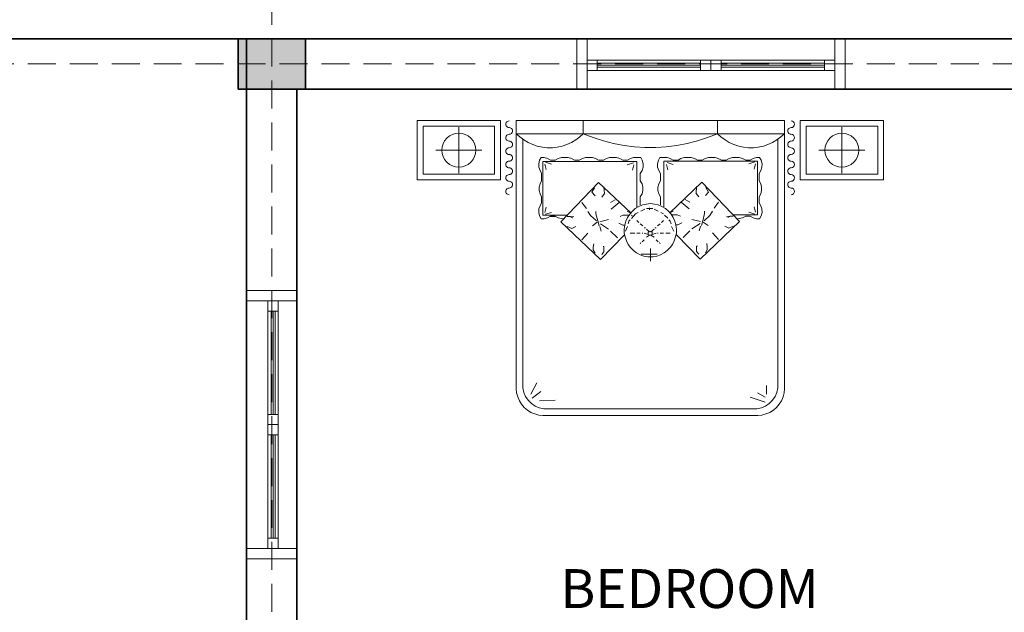
# Model space of a CAD drawing. Units: inches. Extents: x 782 to 2660, y -1008 to 166.
# Tile 8 of 12: x 1058 to 1234, y -58 to 48. Entities that reach past the tile are written whole.
import ezdxf

# ---------------------------------------------------------------- set-up
doc = ezdxf.new("R2010")
doc.units = ezdxf.units.IN
doc.header["$MEASUREMENT"] = 0
doc.linetypes.add('DASHED', pattern=[0.75, 0.5, -0.25])
for name, color, linetype, lineweight in [('A-ANNO-DIMS', 4, 'Continuous', 18), ('A-AREA-IDEN', 4, 'Continuous', 18), ('A-COLS', 7, 'Continuous', 35), ('A-FURN', 8, 'Continuous', 13), ('A-Glaz', 4, 'Continuous', 18), ('A-GRID', 8, 'DASHED', 13), ('A-WALL', 7, 'Continuous', 35)]:
    doc.layers.add(name, color=color, linetype=linetype, lineweight=lineweight)
doc.styles.get("Standard").update_dxf_attribs({"font": 'arial.ttf'})
doc.dimstyles.get("Standard").update_dxf_attribs({"dimtxt": 5, "dimasz": 2, "dimexe": 0.18, "dimexo": 0.0625, "dimgap": 0.09, "dimtad": 0, "dimtih": 1, "dimtoh": 1, "dimdec": 0, "dimzin": 0, "dimdsep": 46, "dimlunit": 3, "dimtxsty": 'Standard', "dimblk": 'ARCHTICK', "dimcen": 0.09, "dimadec": 0, "dimazin": 0, "dimtfac": 1, "dimtdec": 0, "dimtofl": 0, "dimtmove": 0, "dimatfit": 3, "dimfxl": 1, "dimtolj": 1, "dimtzin": 0, "dimarcsym": 0})

# ---------------------------------------------------------------- blocks, each defined once
blk = doc.blocks.new('d-bed-4')
at = {"color": 0, "linetype": 'ByBlock'}
for p, q in [((0.56, 0), (0, 0)), ((0, 0), (0, -0.4)), ((0.56, -0.4), (0.56, 0)), ((0.6639, -1.8), (0.6639, 0)), ((0.6639, 0), (2.4639, 0)), ((0.6639, 0), (2.4639, 0)), ((0.6639, -1.8), (0.6639, 0)), ((1.1139, 0), (1.1139, -0.09)), ((2.0139, 0), (2.0139, -0.09)), ((2.4639, 0), (2.4639, -1.8)), ((2.4639, 0), (2.4639, -1.8)), ((2.5679, -0.4), (2.5679, 0)), ((2.5679, 0), (3.1279, 0)), ((3.1279, 0), (3.1279, -0.4)), ((0.52, -0.04), (0.04, -0.04)), ((0.04, -0.04), (0.04, -0.36)), ((0.28, -0.0461), (0.28, -0.3539)), ((0.52, -0.36), (0.52, -0.04)), ((2.6079, -0.36), (2.6079, -0.04)), ((2.6079, -0.04), (3.0879, -0.04)), ((2.8479, -0.0461), (2.8479, -0.3539)), ((3.0879, -0.04), (3.0879, -0.36)), ((2.4639, -0.09), (0.6639, -0.09)), ((0.6639, -0.09), (0.6891, -0.1116)), ((0.6891, -0.1116), (0.7161, -0.1314)), ((0.7089, -1.7946), (0.7089, -0.1278)), ((0.7161, -0.1314), (0.7449, -0.1476)), ((1.0347, -0.1476), (1.0635, -0.1314)), ((1.0635, -0.1314), (1.0905, -0.1116)), ((1.0905, -0.1116), (1.1139, -0.09)), ((1.1139, -0.09), (1.1805, -0.1152)), ((1.1805, -0.1152), (1.2489, -0.1368)), ((1.8789, -0.1368), (1.9473, -0.1152)), ((1.9473, -0.1152), (2.0139, -0.09)), ((2.0139, -0.09), (2.0373, -0.1116)), ((2.0373, -0.1116), (2.0643, -0.1314)), ((2.0643, -0.1314), (2.0931, -0.1476)), ((2.3829, -0.1476), (2.4117, -0.1314)), ((2.4117, -0.1314), (2.4387, -0.1116)), ((2.4189, -0.1278), (2.4189, -1.7946)), ((2.4387, -0.1116), (2.4639, -0.09)), ((0.7449, -0.1476), (0.7755, -0.162)), ((0.7755, -0.162), (0.8061, -0.1728)), ((0.8061, -0.1728), (0.8403, -0.18)), ((0.8403, -0.18), (0.8727, -0.1836)), ((0.8727, -0.1836), (0.9069, -0.1836)), ((0.9069, -0.1836), (0.9393, -0.18)), ((0.9393, -0.18), (0.9717, -0.1728)), ((0.9717, -0.1728), (1.0041, -0.162)), ((1.0041, -0.162), (1.0347, -0.1476)), ((1.2489, -0.1368), (1.3173, -0.1548)), ((1.3173, -0.1548), (1.3875, -0.1692)), ((1.3875, -0.1692), (1.4577, -0.1782)), ((1.4577, -0.1782), (1.5279, -0.1818)), ((1.5279, -0.1818), (1.5999, -0.1818)), ((1.5999, -0.1818), (1.6701, -0.1782)), ((1.6701, -0.1782), (1.7403, -0.1692)), ((1.7403, -0.1692), (1.8105, -0.1548)), ((1.8105, -0.1548), (1.8789, -0.1368)), ((2.0931, -0.1476), (2.1237, -0.162)), ((2.1237, -0.162), (2.1561, -0.1728)), ((2.1561, -0.1728), (2.1885, -0.18)), ((2.1885, -0.18), (2.2209, -0.1836)), ((2.2209, -0.1836), (2.2551, -0.1836)), ((2.2551, -0.1836), (2.2875, -0.18)), ((2.2875, -0.18), (2.3217, -0.1728)), ((2.3217, -0.1728), (2.3523, -0.162)), ((2.3523, -0.162), (2.3829, -0.1476)), ((0.1261, -0.2), (0.4339, -0.2)), ((0.8205, -0.2682), (0.8313, -0.2484)), ((0.8313, -0.2484), (0.8529, -0.2484)), ((0.8529, -0.2484), (0.8745, -0.2556)), ((0.8745, -0.2556), (0.8943, -0.2664)), ((0.9249, -0.2664), (0.9465, -0.2556)), ((0.9465, -0.2556), (0.9681, -0.2502)), ((0.9681, -0.2502), (0.9897, -0.2484)), ((0.9897, -0.2484), (1.0131, -0.2502)), ((1.0131, -0.2502), (1.0347, -0.2556)), ((1.0347, -0.2556), (1.0563, -0.2664)), ((1.0869, -0.2664), (1.1085, -0.2556)), ((1.1085, -0.2556), (1.1301, -0.2502)), ((1.1301, -0.2502), (1.1517, -0.2484)), ((1.1517, -0.2484), (1.1751, -0.2502)), ((1.1751, -0.2502), (1.1967, -0.2556)), ((1.1967, -0.2556), (1.2165, -0.2664)), ((1.2489, -0.2664), (1.2687, -0.2556)), ((1.2687, -0.2556), (1.2903, -0.2502)), ((1.2903, -0.2502), (1.3137, -0.2484)), ((1.3137, -0.2484), (1.3371, -0.2502)), ((1.3371, -0.2502), (1.3587, -0.2556)), ((1.3587, -0.2556), (1.3785, -0.2664)), ((1.4109, -0.2664), (1.4307, -0.2556)), ((1.4307, -0.2556), (1.4505, -0.2484)), ((1.4505, -0.2484), (1.4739, -0.2484)), ((1.4739, -0.2484), (1.5009, -0.2484)), ((1.5009, -0.2484), (1.5099, -0.2682)), ((1.6269, -0.2484), (1.6179, -0.2682)), ((1.6539, -0.2484), (1.6269, -0.2484)), ((1.6773, -0.2484), (1.6539, -0.2484)), ((1.6971, -0.2556), (1.6773, -0.2484)), ((1.7169, -0.2664), (1.6971, -0.2556)), ((1.7691, -0.2556), (1.7493, -0.2664)), ((1.7907, -0.2502), (1.7691, -0.2556)), ((1.8141, -0.2484), (1.7907, -0.2502)), ((1.8375, -0.2502), (1.8141, -0.2484)), ((1.8591, -0.2556), (1.8375, -0.2502)), ((1.8789, -0.2664), (1.8591, -0.2556)), ((1.9311, -0.2556), (1.9113, -0.2664)), ((1.9527, -0.2502), (1.9311, -0.2556)), ((1.9761, -0.2484), (1.9527, -0.2502)), ((1.9977, -0.2502), (1.9761, -0.2484)), ((2.0193, -0.2556), (1.9977, -0.2502)), ((2.0409, -0.2664), (2.0193, -0.2556)), ((2.0931, -0.2556), (2.0715, -0.2664)), ((2.1147, -0.2502), (2.0931, -0.2556)), ((2.1381, -0.2484), (2.1147, -0.2502)), ((2.1597, -0.2502), (2.1381, -0.2484)), ((2.1813, -0.2556), (2.1597, -0.2502)), ((2.2029, -0.2664), (2.1813, -0.2556)), ((2.2533, -0.2556), (2.2335, -0.2664)), ((2.2749, -0.2484), (2.2533, -0.2556)), ((2.2965, -0.2484), (2.2749, -0.2484)), ((2.3073, -0.2682), (2.2965, -0.2484)), ((3.0018, -0.2), (2.6939, -0.2)), ((0.8151, -0.2916), (0.8205, -0.2682)), ((0.8169, -0.315), (0.8151, -0.2916)), ((0.8241, -0.3366), (0.8169, -0.315)), ((0.8439, -0.6354), (0.8439, -0.2754)), ((0.8439, -0.2754), (1.4721, -0.2754)), ((0.8565, -0.2934), (0.8655, -0.3294)), ((0.8619, -0.2808), (0.9015, -0.2934)), ((0.8943, -0.2664), (0.9249, -0.2664)), ((1.0563, -0.2664), (1.0869, -0.2664)), ((1.2165, -0.2664), (1.2489, -0.2664)), ((1.3785, -0.2664), (1.4109, -0.2664)), ((1.4505, -0.2844), (1.4091, -0.2988)), ((1.4541, -0.2988), (1.4451, -0.3348)), ((1.4721, -0.2754), (1.4721, -0.5814)), ((1.5153, -0.315), (1.5081, -0.3366)), ((1.5099, -0.2682), (1.5153, -0.2916)), ((1.5153, -0.2916), (1.5153, -0.315)), ((1.6179, -0.2682), (1.6125, -0.2916)), ((1.6125, -0.2916), (1.6125, -0.315)), ((1.6125, -0.315), (1.6197, -0.3366)), ((2.2821, -0.2736), (1.6539, -0.2736)), ((1.6539, -0.2736), (1.6539, -0.5796)), ((1.6719, -0.297), (1.6809, -0.333)), ((1.6755, -0.2826), (1.7169, -0.297)), ((1.7493, -0.2664), (1.7169, -0.2664)), ((1.9113, -0.2664), (1.8789, -0.2664)), ((2.0715, -0.2664), (2.0409, -0.2664)), ((2.2335, -0.2664), (2.2029, -0.2664)), ((2.2641, -0.279), (2.2245, -0.2916)), ((2.2695, -0.2916), (2.2605, -0.3276)), ((2.2821, -0.6336), (2.2821, -0.2736)), ((2.3037, -0.3366), (2.3109, -0.315)), ((2.3127, -0.2916), (2.3073, -0.2682)), ((2.3109, -0.315), (2.3127, -0.2916)), ((0.04, -0.36), (0.52, -0.36)), ((0.8349, -0.3564), (0.8241, -0.3366)), ((0.8349, -0.405), (0.8349, -0.3564)), ((1.5081, -0.3366), (1.4955, -0.3564)), ((1.4955, -0.3564), (1.4955, -0.405)), ((1.6197, -0.3366), (1.6323, -0.3564)), ((1.6323, -0.3564), (1.6323, -0.405)), ((2.2929, -0.3564), (2.3037, -0.3366)), ((2.2929, -0.405), (2.2929, -0.3564)), ((3.0879, -0.36), (2.6079, -0.36)), ((0, -0.4), (0.56, -0.4)), ((0.8187, -0.4482), (0.8241, -0.4248)), ((0.8187, -0.4698), (0.8187, -0.4482)), ((0.8241, -0.4248), (0.8349, -0.405)), ((0.9645, -0.6804), (1.2165, -0.4158)), ((1.1895, -0.4518), (1.1715, -0.4824)), ((1.2165, -0.4158), (1.4325, -0.621)), ((1.2525, -0.4464), (1.2561, -0.4914)), ((1.4955, -0.405), (1.5081, -0.4248)), ((1.5081, -0.4248), (1.5135, -0.4482)), ((1.5135, -0.4482), (1.5135, -0.4698)), ((1.6197, -0.4248), (1.6143, -0.4482)), ((1.6143, -0.4482), (1.6143, -0.4698)), ((1.6323, -0.405), (1.6197, -0.4248)), ((1.9095, -0.414), (1.6935, -0.6192)), ((1.8735, -0.4446), (1.8699, -0.4896)), ((2.1615, -0.6786), (1.9095, -0.414)), ((1.9365, -0.45), (1.9545, -0.4806)), ((2.3037, -0.4248), (2.2929, -0.405)), ((2.3091, -0.4482), (2.3037, -0.4248)), ((2.3091, -0.4698), (2.3091, -0.4482)), ((3.1279, -0.4), (2.5679, -0.4)), ((0.8241, -0.4932), (0.8187, -0.4698)), ((0.8349, -0.513), (0.8241, -0.4932)), ((0.8349, -0.5526), (0.8349, -0.513)), ((1.1715, -0.4824), (1.1931, -0.5058)), ((1.2561, -0.4914), (1.2381, -0.5148)), ((1.5081, -0.4932), (1.4955, -0.513)), ((1.4955, -0.513), (1.4955, -0.567)), ((1.5135, -0.4698), (1.5081, -0.4932)), ((1.6143, -0.4698), (1.6197, -0.4932)), ((1.6197, -0.4932), (1.6323, -0.513)), ((1.6323, -0.513), (1.6323, -0.567)), ((1.8699, -0.4896), (1.8879, -0.513)), ((1.9545, -0.4806), (1.9329, -0.504)), ((2.2929, -0.513), (2.3037, -0.4932)), ((2.2929, -0.5526), (2.2929, -0.513)), ((2.3037, -0.4932), (2.3091, -0.4698)), ((0.8151, -0.6174), (0.8169, -0.594)), ((0.8169, -0.594), (0.8241, -0.5724)), ((0.8241, -0.5724), (0.8349, -0.5526)), ((0.8565, -0.6174), (0.8655, -0.5814)), ((1.1049, -0.5508), (1.1355, -0.5904)), ((1.3281, -0.5328), (1.2975, -0.5508)), ((1.3551, -0.5508), (1.3011, -0.5958)), ((1.4433, -0.6102), (1.4631, -0.5922)), ((1.4631, -0.5922), (1.4865, -0.5778)), ((1.4865, -0.5778), (1.5117, -0.567)), ((1.5117, -0.567), (1.5369, -0.5616)), ((1.5369, -0.5616), (1.5639, -0.558)), ((1.5369, -0.5904), (1.5621, -0.5904)), ((1.5801, -0.5904), (1.5549, -0.5904)), ((1.5585, -0.5868), (1.5585, -0.5994)), ((1.5585, -0.5868), (1.5585, -0.5994)), ((1.5639, -0.558), (1.5909, -0.5616)), ((1.5909, -0.5616), (1.6161, -0.567)), ((1.6161, -0.567), (1.6413, -0.5778)), ((1.6413, -0.5778), (1.6647, -0.5922)), ((1.6647, -0.5922), (1.6845, -0.6102)), ((1.7709, -0.549), (1.8249, -0.594)), ((1.7979, -0.531), (1.8285, -0.549)), ((2.0211, -0.549), (1.9905, -0.5886)), ((2.2695, -0.6156), (2.2605, -0.5796)), ((2.3037, -0.5724), (2.2929, -0.5526)), ((2.3109, -0.594), (2.3037, -0.5724)), ((2.3127, -0.6174), (2.3109, -0.594)), ((0.8205, -0.6408), (0.8151, -0.6174)), ((0.8313, -0.6606), (0.8205, -0.6408)), ((1.0095, -0.6354), (0.8439, -0.6354)), ((0.8745, -0.6534), (0.8529, -0.6606)), ((0.8619, -0.63), (0.9015, -0.6174)), ((0.8943, -0.6426), (0.8745, -0.6534)), ((0.9069, -0.6444), (0.8925, -0.6444)), ((0.9249, -0.6426), (0.8943, -0.6426)), ((0.9159, -0.6444), (0.9069, -0.6444)), ((0.9249, -0.6444), (0.9159, -0.6444)), ((0.9465, -0.6534), (0.9249, -0.6426)), ((0.9681, -0.6588), (0.9465, -0.6534)), ((0.9825, -0.6606), (0.9681, -0.6588)), ((1.0059, -0.6444), (1.0239, -0.6444)), ((1.0239, -0.6444), (1.0419, -0.6534)), ((1.0419, -0.6534), (1.0275, -0.6444)), ((1.0275, -0.6444), (1.0509, -0.648)), ((1.1625, -0.639), (1.1445, -0.612)), ((1.2021, -0.675), (1.1625, -0.639)), ((1.1985, -0.6264), (1.1985, -0.612)), ((1.2111, -0.675), (1.1985, -0.6264)), ((1.3821, -0.6354), (1.3605, -0.6444)), ((1.4145, -0.6354), (1.3821, -0.6354)), ((1.4001, -0.6768), (1.4109, -0.6516)), ((1.4091, -0.612), (1.4325, -0.621)), ((1.4109, -0.6516), (1.4253, -0.63)), ((1.4145, -0.6354), (1.4181, -0.639)), ((1.4253, -0.63), (1.4433, -0.6102)), ((1.4649, -0.6264), (1.4379, -0.6588)), ((1.4379, -0.6354), (1.4415, -0.6408)), ((1.4649, -0.6264), (1.4829, -0.6174)), ((1.5279, -0.5958), (1.5009, -0.6084)), ((1.5891, -0.5958), (1.6161, -0.6084)), ((1.6521, -0.6264), (1.6341, -0.6174)), ((1.6593, -0.6354), (1.6809, -0.657)), ((1.6845, -0.6102), (1.7025, -0.63)), ((1.7169, -0.6102), (1.6935, -0.6192)), ((1.7025, -0.63), (1.7169, -0.6516)), ((1.7115, -0.6336), (1.7079, -0.6372)), ((1.7115, -0.6336), (1.7439, -0.6336)), ((1.7169, -0.6516), (1.7277, -0.6768)), ((1.7439, -0.6336), (1.7655, -0.6426)), ((1.9149, -0.6732), (1.9275, -0.6246)), ((1.9239, -0.6732), (1.9635, -0.6372)), ((1.9275, -0.6246), (1.9275, -0.6102)), ((1.9635, -0.6372), (1.9815, -0.6102)), ((2.0985, -0.6426), (2.0751, -0.6462)), ((2.1021, -0.6426), (2.0841, -0.6516)), ((2.0841, -0.6516), (2.0985, -0.6426)), ((2.1201, -0.6426), (2.1021, -0.6426)), ((2.1165, -0.6336), (2.2821, -0.6336)), ((2.1453, -0.6606), (2.1597, -0.6588)), ((2.1597, -0.6588), (2.1813, -0.6534)), ((2.1813, -0.6534), (2.2029, -0.6426)), ((2.2011, -0.6426), (2.2101, -0.6426)), ((2.2029, -0.6426), (2.2335, -0.6426)), ((2.2101, -0.6426), (2.2191, -0.6426)), ((2.2191, -0.6426), (2.2335, -0.6426)), ((2.2641, -0.6282), (2.2245, -0.6156)), ((2.2335, -0.6426), (2.2533, -0.6534)), ((2.2533, -0.6534), (2.2749, -0.6606)), ((2.2965, -0.6606), (2.3073, -0.6408)), ((2.3073, -0.6408), (2.3127, -0.6174)), ((0.8529, -0.6606), (0.8313, -0.6606)), ((1.2291, -0.9324), (0.9645, -0.6804)), ((1.0059, -0.711), (1.0365, -0.7254)), ((1.0365, -0.7254), (1.0545, -0.7164)), ((1.0545, -0.7164), (1.0635, -0.711)), ((1.1751, -0.7074), (1.2075, -0.684)), ((1.2201, -0.7074), (1.2111, -0.675)), ((1.2255, -0.6804), (1.2831, -0.666)), ((1.2255, -0.711), (1.2345, -0.7434)), ((1.2291, -0.693), (1.2831, -0.729)), ((1.3785, -0.702), (1.3515, -0.6894)), ((1.3785, -0.702), (1.3911, -0.702)), ((1.3893, -0.729), (1.3929, -0.702)), ((1.3929, -0.702), (1.4001, -0.6768)), ((1.3965, -0.7434), (1.4109, -0.711)), ((1.4199, -0.6768), (1.4145, -0.6948)), ((1.4199, -0.6768), (1.4289, -0.6678)), ((1.4865, -0.6858), (1.4739, -0.6714)), ((1.5135, -0.7074), (1.4955, -0.6948)), ((1.5315, -0.72), (1.5225, -0.72)), ((1.5945, -0.72), (1.6035, -0.72)), ((1.6125, -0.7074), (1.6305, -0.6948)), ((1.6395, -0.6858), (1.6521, -0.6714)), ((1.6971, -0.6768), (1.6881, -0.6678)), ((1.6971, -0.6768), (1.7025, -0.6948)), ((1.7205, -0.7434), (1.7061, -0.711)), ((1.7277, -0.6768), (1.7349, -0.702)), ((1.7475, -0.7002), (1.7349, -0.7002)), ((1.7349, -0.702), (1.7385, -0.729)), ((1.7475, -0.7002), (1.7745, -0.6876)), ((1.9005, -0.6786), (1.8429, -0.6642)), ((1.8969, -0.6912), (1.8429, -0.7272)), ((1.9005, -0.7092), (1.8915, -0.7416)), ((1.8969, -0.9306), (2.1615, -0.6786)), ((1.9059, -0.7056), (1.9149, -0.6732)), ((1.9509, -0.7056), (1.9185, -0.6822)), ((2.0715, -0.7146), (2.0625, -0.7092)), ((2.0895, -0.7236), (2.0715, -0.7146)), ((2.1201, -0.7092), (2.0895, -0.7236)), ((2.2749, -0.6606), (2.2965, -0.6606)), ((1.1049, -0.801), (1.1445, -0.756)), ((1.2291, -0.9324), (1.3875, -0.7704)), ((1.3425, -0.7884), (1.2975, -0.7434)), ((1.3893, -0.756), (1.3893, -0.729)), ((1.3947, -0.7812), (1.3893, -0.756)), ((1.4037, -0.8082), (1.3947, -0.7812)), ((1.4595, -0.756), (1.4289, -0.756)), ((1.4955, -0.756), (1.4739, -0.756)), ((1.5135, -0.756), (1.5099, -0.756)), ((1.5495, -0.765), (1.5225, -0.756)), ((1.5315, -0.792), (1.5315, -0.792)), ((1.5585, -0.747), (1.5369, -0.729)), ((1.5585, -0.7704), (1.5369, -0.783)), ((1.5495, -0.756), (1.5495, -0.747)), ((1.5495, -0.747), (1.5585, -0.747)), ((1.5495, -0.765), (1.5495, -0.756)), ((1.5585, -0.7704), (1.5495, -0.765)), ((1.5585, -0.747), (1.5621, -0.7452)), ((1.5585, -0.7704), (1.5621, -0.7704)), ((1.5675, -0.747), (1.5621, -0.7452)), ((1.5675, -0.7704), (1.5621, -0.7704)), ((1.5675, -0.747), (1.5891, -0.729)), ((1.5765, -0.747), (1.5675, -0.747)), ((1.5675, -0.7704), (1.5765, -0.765)), ((1.5675, -0.7704), (1.5891, -0.783)), ((1.5765, -0.756), (1.5765, -0.747)), ((1.5765, -0.765), (1.5765, -0.756)), ((1.5765, -0.765), (1.6035, -0.756)), ((1.5945, -0.792), (1.5945, -0.792)), ((1.6125, -0.756), (1.6161, -0.756)), ((1.6305, -0.756), (1.6521, -0.756)), ((1.6665, -0.756), (1.6971, -0.756)), ((1.7331, -0.7812), (1.7241, -0.8082)), ((1.7385, -0.756), (1.7331, -0.7812)), ((1.7385, -0.729), (1.7385, -0.756)), ((1.8969, -0.9306), (1.7385, -0.7686)), ((1.7835, -0.7866), (1.8285, -0.7416)), ((2.0211, -0.7992), (1.9815, -0.7542)), ((1.1805, -0.8514), (1.1841, -0.828)), ((1.1805, -0.8694), (1.1805, -0.8514)), ((1.2525, -0.846), (1.2471, -0.846)), ((1.2525, -0.882), (1.2525, -0.846)), ((1.4145, -0.8316), (1.4037, -0.8082)), ((1.4307, -0.8532), (1.4145, -0.8316)), ((1.4505, -0.873), (1.4307, -0.8532)), ((1.5009, -0.819), (1.4955, -0.828)), ((1.5225, -0.801), (1.5099, -0.8154)), ((1.6035, -0.801), (1.6161, -0.8154)), ((1.6251, -0.819), (1.6305, -0.828)), ((1.6971, -0.8532), (1.6773, -0.873)), ((1.7133, -0.8316), (1.6971, -0.8532)), ((1.7241, -0.8082), (1.7133, -0.8316)), ((1.8735, -0.8802), (1.8735, -0.8442)), ((1.8735, -0.8442), (1.8789, -0.8442)), ((1.9455, -0.8496), (1.9419, -0.8262)), ((1.9455, -0.8676), (1.9455, -0.8496)), ((1.1931, -0.891), (1.1805, -0.8694)), ((1.2381, -0.9), (1.2525, -0.882)), ((1.4703, -0.8892), (1.4505, -0.873)), ((1.4955, -0.9018), (1.4703, -0.8892)), ((1.5207, -0.9108), (1.4955, -0.9018)), ((1.6089, -0.8964), (1.5027, -0.8964)), ((1.5459, -0.9162), (1.5207, -0.9108)), ((1.5639, -0.9162), (1.5459, -0.9162)), ((1.5639, -0.945), (1.5639, -0.8604)), ((1.5819, -0.9162), (1.5639, -0.9162)), ((1.6071, -0.9108), (1.5819, -0.9162)), ((1.6323, -0.9018), (1.6071, -0.9108)), ((1.6575, -0.8892), (1.6323, -0.9018)), ((1.6773, -0.873), (1.6575, -0.8892)), ((1.8879, -0.8982), (1.8735, -0.8802)), ((1.9329, -0.8892), (1.9455, -0.8676)), ((0.7629, -1.836), (0.8025, -1.7604)), ((2.3415, -1.836), (2.3415, -1.7784)), ((0.6675, -1.827), (0.6639, -1.8)), ((0.6675, -1.827), (0.6639, -1.8)), ((0.6747, -1.854), (0.6675, -1.827)), ((0.6747, -1.854), (0.6675, -1.827)), ((0.7161, -1.8252), (0.7089, -1.7946)), ((0.7269, -1.8522), (0.7161, -1.8252)), ((0.7719, -1.863), (0.8295, -1.818)), ((2.3325, -1.8576), (2.2821, -1.827)), ((2.4117, -1.8252), (2.4009, -1.8522)), ((2.4189, -1.7946), (2.4117, -1.8252)), ((2.4603, -1.827), (2.4531, -1.854)), ((2.4603, -1.827), (2.4531, -1.854)), ((2.4639, -1.8), (2.4603, -1.827)), ((2.4639, -1.8), (2.4603, -1.827)), ((0.6855, -1.881), (0.6747, -1.854)), ((0.6855, -1.881), (0.6747, -1.854)), ((0.6999, -1.9044), (0.6855, -1.881)), ((0.6999, -1.9044), (0.6855, -1.881)), ((0.7179, -1.926), (0.6999, -1.9044)), ((0.7179, -1.926), (0.6999, -1.9044)), ((0.7449, -1.8774), (0.7269, -1.8522)), ((0.7665, -1.899), (0.7449, -1.8774)), ((0.7917, -1.917), (0.7665, -1.899)), ((0.8205, -1.881), (0.9249, -1.8756)), ((2.3325, -1.89), (2.2335, -1.8576)), ((2.3613, -1.899), (2.3361, -1.917)), ((2.3829, -1.8774), (2.3613, -1.899)), ((2.4009, -1.8522), (2.3829, -1.8774)), ((2.4279, -1.9044), (2.4099, -1.926)), ((2.4279, -1.9044), (2.4099, -1.926)), ((2.4423, -1.881), (2.4279, -1.9044)), ((2.4423, -1.881), (2.4279, -1.9044)), ((2.4531, -1.854), (2.4423, -1.881)), ((2.4531, -1.854), (2.4423, -1.881)), ((0.7395, -1.944), (0.7179, -1.926)), ((0.7395, -1.944), (0.7179, -1.926)), ((0.7629, -1.9584), (0.7395, -1.944)), ((0.7629, -1.9584), (0.7395, -1.944)), ((0.7899, -1.9692), (0.7629, -1.9584)), ((0.7899, -1.9692), (0.7629, -1.9584)), ((0.8169, -1.9764), (0.7899, -1.9692)), ((0.8169, -1.9764), (0.7899, -1.9692)), ((0.8187, -1.9278), (0.7917, -1.917)), ((0.8439, -1.98), (0.8169, -1.9764)), ((0.8439, -1.98), (0.8169, -1.9764)), ((0.8493, -1.935), (0.8187, -1.9278)), ((2.2839, -1.98), (0.8439, -1.98)), ((2.2839, -1.98), (0.8439, -1.98)), ((2.2785, -1.935), (0.8493, -1.935)), ((2.3091, -1.9278), (2.2785, -1.935)), ((2.3109, -1.9764), (2.2839, -1.98)), ((2.3109, -1.9764), (2.2839, -1.98)), ((2.3361, -1.917), (2.3091, -1.9278)), ((2.3379, -1.9692), (2.3109, -1.9764)), ((2.3379, -1.9692), (2.3109, -1.9764)), ((2.3649, -1.9584), (2.3379, -1.9692)), ((2.3649, -1.9584), (2.3379, -1.9692)), ((2.3883, -1.944), (2.3649, -1.9584)), ((2.3883, -1.944), (2.3649, -1.9584)), ((2.4099, -1.926), (2.3883, -1.944)), ((2.4099, -1.926), (2.3883, -1.944))]:
    blk.add_line(p, q, dxfattribs=at)
for centre, major_axis, start_param, end_param in [((0.6172, -0.0263), (-0.0159, 0.0159), 5.497787, 8.63938), ((0.6172, -0.0713), (-0.0159, 0.0159), 2.356194, 5.497787), ((2.5072, -0.0713), (0.0159, 0.0159), 0.785398, 3.926991), ((2.5072, -0.0263), (0.0159, 0.0159), 3.926991, 7.068583), ((0.6172, -0.1163), (-0.0159, 0.0159), 5.497787, 8.63938), ((2.5072, -0.1163), (0.0159, 0.0159), 3.926991, 7.068583), ((0.6172, -0.2063), (-0.0159, 0.0159), 5.497787, 8.63938), ((0.6172, -0.1613), (-0.0159, 0.0159), 2.356194, 5.497787), ((0.6172, -0.1613), (-0.0159, 0.0159), 2.356194, 5.497787), ((2.5072, -0.1613), (0.0159, 0.0159), 0.785398, 3.926991), ((2.5072, -0.1613), (0.0159, 0.0159), 0.785398, 3.926991), ((2.5072, -0.2063), (0.0159, 0.0159), 3.926991, 7.068583), ((0.6172, -0.2513), (-0.0159, 0.0159), 2.356194, 5.497787), ((2.5072, -0.2513), (0.0159, 0.0159), 0.785398, 3.926991), ((0.6172, -0.2963), (-0.0159, 0.0159), 5.497787, 8.63938), ((0.6172, -0.3413), (-0.0159, 0.0159), 2.356194, 5.497787), ((2.5072, -0.3413), (0.0159, 0.0159), 0.785398, 3.926991), ((2.5072, -0.2963), (0.0159, 0.0159), 3.926991, 7.068583), ((0.6172, -0.3863), (-0.0159, 0.0159), 5.497787, 8.63938), ((2.5072, -0.3863), (0.0159, 0.0159), 3.926991, 7.068583), ((0.6172, -0.4763), (-0.0159, 0.0159), 5.497787, 8.63938), ((0.6172, -0.4313), (-0.0159, 0.0159), 2.356194, 5.497787), ((2.5072, -0.4313), (0.0159, 0.0159), 0.785398, 3.926991), ((2.5072, -0.4763), (0.0159, 0.0159), 3.926991, 7.068583)]:
    blk.add_ellipse(centre, major_axis=major_axis, ratio=1, start_param=start_param, end_param=end_param, dxfattribs=at)
for centre in [(0.28, -0.2), (2.8479, -0.2)]:
    blk.add_ellipse(centre, major_axis=(-0.0806, 0.0806), ratio=1, dxfattribs=at)
blk = doc.blocks.new('WIN-48-FRAME-A')
for p, q in [((0, 48), (0, 0)), ((0, 48), (9, 48)), ((9, 48), (0, 48)), ((9, 48), (9, 0)), ((9, 46.15), (0, 46.15)), ((9, 46.15), (0, 46.15)), ((9, 46.15), (0, 46.15)), ((3.35, 1.85), (3.35, 46.15)), ((5.19, 1.85), (5.19, 46.15)), ((5.19, 44.31), (3.35, 44.31)), ((3.9, 44.31), (3.9, 25.85)), ((4.27, 44.31), (4.27, 25.85)), ((4.64, 44.31), (4.64, 25.85)), ((3.35, 25.85), (5.19, 25.85)), ((3.35, 24), (5.19, 24)), ((3.35, 22.15), (5.19, 22.15)), ((3.9, 3.69), (3.9, 22.15)), ((4.27, 3.69), (4.27, 22.15)), ((4.64, 3.69), (4.64, 22.15)), ((5.19, 3.69), (3.35, 3.69)), ((9, 1.85), (0, 1.85)), ((9, 1.85), (0, 1.85)), ((0, 0), (9, 0)), ((0, 0), (9, 0))]:
    blk.add_line(p, q)
blk = doc.blocks.new('COL-9X12')
h = blk.add_hatch(color=256)
h.dxf.hatch_style = 1
h.paths.add_polyline_path([(9, 12), (0, 12), (0, 0), (9, 0)])
blk.add_lwpolyline([(0, 12), (9, 12), (9, 0), (0, 0)], close=True)
blk = doc.blocks.new('_ArchTick')
at = {"color": 0, "linetype": 'ByBlock', "const_width": 0.15}
blk.add_lwpolyline([(-0.5, -0.5), (0.5, 0.5)], dxfattribs=at)
blk = doc.blocks.new('*D52')
at = {"layer": 'A-ANNO-DIMS', "color": 0, "lineweight": -2, "transparency": 16777216}
for p, q in [((982.68, 45.07), (982.68, 163.27)), ((982.68, 163.09), (1186.01, 163.09)), ((1406.68, 163.09), (1203.36, 163.09)), ((1406.68, 45.07), (1406.68, 163.27))]:
    blk.add_line(p, q, dxfattribs=at)
at = {"layer": 'Defpoints', "color": 0, "transparency": 16777216}
for p in [(1406.68, 163.09), (982.68, 45.01), (1406.68, 45.01)]:
    blk.add_point(p, dxfattribs=at)
at = {"layer": 'A-ANNO-DIMS', "color": 0, "lineweight": -2, "transparency": 16777216, "xscale": 2, "yscale": 2, "zscale": 2, "rotation": 180}
blk.add_blockref('_ArchTick', (982.68, 163.09), dxfattribs=at)
at = {"layer": 'A-ANNO-DIMS', "color": 0, "lineweight": -2, "transparency": 16777216, "xscale": 2, "yscale": 2, "zscale": 2}
blk.add_blockref('_ArchTick', (1406.68, 163.09), dxfattribs=at)
at = {"layer": 'A-ANNO-DIMS', "color": 0, "transparency": 16777216, "insert": (1194.68, 163.09), "char_height": 5, "attachment_point": 5}
blk.add_mtext('\\A1;35\'-4"', dxfattribs=at)

msp = doc.modelspace()

# ---------------------------------------------------------------- linework, layer by layer
at = {"layer": 'A-Glaz'}
for p, q in [((1107.68, 0.01), (1098.68, 0.01)), ((1098.68, 0.01), (1098.68, -1.84)), ((1107.68, 0.01), (1098.68, 0.01)), ((1107.68, -47.99), (1107.68, 0.01)), ((1107.68, -1.84), (1107.68, 0.01)), ((1098.68, -1.84), (1107.68, -1.84)), ((1098.68, -1.84), (1107.68, -1.84)), ((1098.68, -46.15), (1098.68, -1.84)), ((1102.49, -1.84), (1102.49, -46.15)), ((1104.34, -1.84), (1104.34, -46.15)), ((1102.49, -3.69), (1104.34, -3.69)), ((1103.04, -3.69), (1103.04, -22.15)), ((1103.41, -3.69), (1103.41, -22.15)), ((1103.78, -3.69), (1103.78, -22.15)), ((1104.34, -22.15), (1102.49, -22.15)), ((1104.34, -23.99), (1102.49, -23.99)), ((1104.34, -25.84), (1102.49, -25.84)), ((1103.04, -44.3), (1103.04, -25.84)), ((1103.41, -44.3), (1103.41, -25.84)), ((1103.78, -44.3), (1103.78, -25.84)), ((1102.49, -44.3), (1104.34, -44.3)), ((1098.68, -46.15), (1107.68, -46.15)), ((1098.68, -47.99), (1098.68, -46.15)), ((1098.68, -46.15), (1107.68, -46.15)), ((1098.68, -46.15), (1107.68, -46.15)), ((1107.68, -46.15), (1107.68, -47.99)), ((1107.68, -47.99), (1098.68, -47.99)), ((1098.68, -47.99), (1107.68, -47.99))]:
    msp.add_line(p, q, dxfattribs=at)
at = {"layer": 'A-GRID', "ltscale": 10}
for p, q in [((1103.18, 82.53), (1103.18, -946.37)), ((1499.56, 40.51), (955.26, 40.51))]:
    msp.add_line(p, q, dxfattribs=at)
at = {"layer": 'A-WALL'}
for p, q in [((982.68, 45.01), (1406.68, 45.01)), ((1098.68, 45.01), (1098.68, -175.99)), ((1107.68, 36.01), (1107.68, -83.99)), ((1107.68, 36.01), (1255.68, 36.01))]:
    msp.add_line(p, q, dxfattribs=at)

# ---------------------------------------------------------------- block references
at = {"layer": 'A-COLS', "rotation": 270.0000000000027}
msp.add_blockref('COL-9X12', (1097.18, 45.01), dxfattribs=at)
at = {"layer": 'A-FURN', "xscale": 26.66666775212405, "yscale": 26.66666775212405, "zscale": 26.66666775212405}
msp.add_blockref('d-bed-4', (1129.15, 30.43), dxfattribs=at)
at = {"layer": 'A-Glaz', "rotation": 90.00000000000036}
msp.add_blockref('WIN-48-FRAME-A', (1205.68, 36.01), dxfattribs=at)

# ---------------------------------------------------------------- texts
at = {"layer": 'A-AREA-IDEN'}
msp.add_text('BEDROOM', height=6.958, dxfattribs=at).set_placement((1154.78, -56.79))

# ---------------------------------------------------------------- dimensions: what is measured, and where the dimension line sits
at = {"layer": 'A-ANNO-DIMS'}
dim = msp.add_linear_dim(base=(1406.68, 163.09), p1=(982.68, 45.01), p2=(1406.68, 45.01), dimstyle='Standard', override={"dimdec": 1, "dimlfac": 1, "dimrnd": 0, "dimzin": 1, "dimdsep": 46, "dimlunit": 4, "dimfrac": 2}, dxfattribs=at)
dim.commit()
dim.dimension.update_dxf_attribs({"geometry": '*D52', "text_midpoint": (1194.68, 163.09)})

doc.saveas('drawing.dxf')
